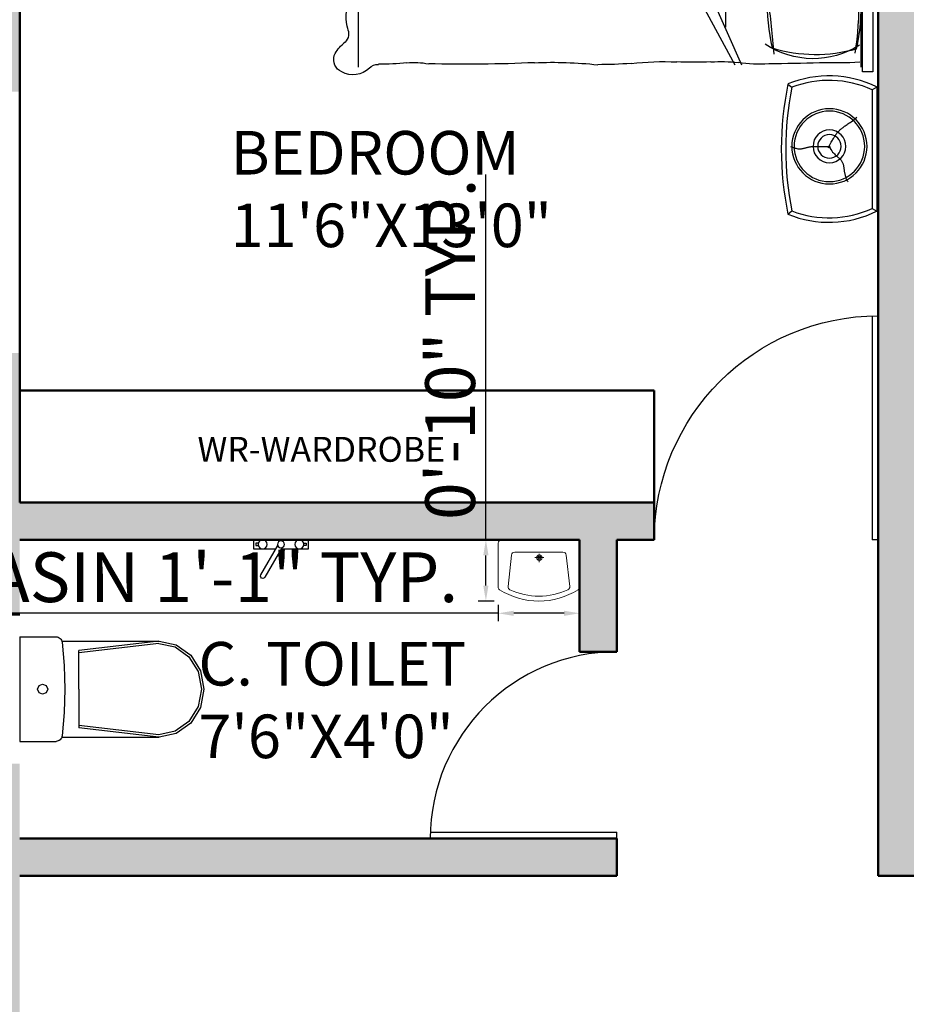
# Model space of a CAD drawing. Units: inches. Extents: x 1986 to 21484, y -1816 to 2016.
# Tile 7 of 85: x 2087 to 2230, y 1607 to 1765. Entities that reach past the tile are written whole.
import ezdxf

# ---------------------------------------------------------------- set-up
doc = ezdxf.new("R2010")
doc.units = ezdxf.units.IN
for name, color, linetype, lineweight in [('A-ANNO-DIMS', 2, 'Continuous', 18), ('A-ANNO-TEXT', 7, 'Continuous', 18), ('A-AREA-IDEN', 3, 'Continuous', 18), ('A-DOOR', 3, 'Continuous', 25), ('A-FLOR-FIXT', 8, 'Continuous', 18), ('A-FURN', 8, 'Continuous', 18), ('A-WALL', 7, 'Continuous', 50), ('A-WALL-PATT', 8, 'Continuous', 13)]:
    doc.layers.add(name, color=color, linetype=linetype, lineweight=lineweight)
doc.layers.add('SANTEH', color=7, linetype='Continuous')
doc.layers.add('TEFRİŞ', color=11, linetype='Continuous')
doc.styles.get("Standard").update_dxf_attribs({"font": 'arial.ttf'})
doc.dimstyles.new('ISO-25', dxfattribs={"dimtxt": 8, "dimasz": 2.5, "dimexe": 1.25, "dimexo": 0.625, "dimtad": 1, "dimdec": 1, "dimlunit": 3, "dimtxsty": 'Standard', "dimcen": 2.5, "dimadec": 0, "dimazin": 0, "dimtfac": 1, "dimtdec": 1, "dimtmove": 0, "dimatfit": 3, "dimfxl": 1, "dimarcsym": 0})

# ---------------------------------------------------------------- blocks, each defined once
blk = doc.blocks.new('D2')
for p, q in [((1722.5, 1505.46), (1722.5, 1475.46)), ((1723.5, 1505.46), (1723.5, 1475.46)), ((1722.5, 1475.46), (1723.5, 1475.46))]:
    blk.add_line(p, q)
blk.add_arc((1722.5, 1475.46), 30, 0, 90)
blk = doc.blocks.new('D1')
for p, q in [((1805.96, 1500.36), (1805.96, 1464.36)), ((1806.96, 1500.36), (1806.96, 1464.36)), ((1805.96, 1464.36), (1806.96, 1464.36))]:
    blk.add_line(p, q)
blk.add_arc((1805.96, 1464.36), 36, 0, 90)
blk = doc.blocks.new('WC 2 Symb_109')
at = {"layer": 'SANTEH'}
for p, q in [((0, 0), (0, 380)), ((0, 380), (132.4, 380)), ((153.6, 364.9), (506.8, 364.9)), ((506.3, 364.9), (215.7, 330.9)), ((506.3, 356), (215.7, 322)), ((215.7, 190), (215.7, 330.9)), ((215.7, 190), (215.7, 49.1)), ((506.3, 24), (215.7, 58)), ((506.3, 15.1), (215.7, 49.1)), ((153.8, 15.1), (506.8, 15.1)), ((0, 0), (132.4, 0))]:
    blk.add_line(p, q, dxfattribs=at)
for points in [[(154.6, 360.1), (153.9, 364.1), (152.3, 367.9), (150.2, 371.3), (147.4, 374.3), (144.1, 376.7), (140.5, 378.5), (136.5, 379.6), (132.4, 380)], [(154.6, 19.7), (158.6, 62.1), (161.4, 104.7), (163.1, 147.3), (163.7, 189.9), (163.1, 232.5), (161.4, 275.1), (158.6, 317.7), (154.6, 360.1)], [(506.8, 15.1), (569.2, 28.4), (622.2, 66.3), (657.6, 123.1), (670, 190), (657.6, 256.9), (622.2, 313.7), (569.2, 351.6), (506.8, 364.9)], [(506.3, 24), (565.5, 36.6), (615.7, 72.6), (649.2, 126.5), (661, 190), (649.2, 253.5), (615.7, 307.4), (565.5, 343.4), (506.3, 356)], [(132.4, 0), (136.5, 0.4), (140.4, 1.5), (144.1, 3.2), (147.3, 5.6), (150.1, 8.6), (152.3, 12), (153.8, 15.7), (154.6, 19.7)]]:
    blk.add_lwpolyline(points, dxfattribs=at)
blk.add_lwpolyline([(83.6, 208.5), (70.4, 203.1), (64.9, 190), (70.4, 176.9), (83.6, 171.5), (96.8, 176.9), (102.2, 190), (96.8, 203.1)], close=True, dxfattribs=at)
blk = doc.blocks.new('A$C2EBB240D')
for p, q in [((480, 375.8), (20, 375.8)), ((0, 355.8), (0, 86.6)), ((500, 355.8), (500, 86.6)), ((60.8, 89.8), (82.3, 282.2)), ((250, 300), (102.1, 300)), ((250, 300), (397.9, 300)), ((439.2, 89.8), (417.7, 282.2))]:
    blk.add_line(p, q)
for points in [[(275.2, 266.4), (219.4, 266.4)], [(247.3, 238.5), (247.3, 288.9)]]:
    blk.add_lwpolyline(points)
for centre, radius, start, end in [((20, 355.8), 20, 90, 180), ((480, 355.8), 20, 0, 90), ((102.1, 280), 20, 90, 173.64284), ((247.3, 266.4), 16.7, 90, 270), ((247.3, 266.4), 10, 90, 270), ((247.3, 266.4), 16.7, 270, 90), ((247.3, 266.4), 10, 270, 90), ((397.9, 280), 20, 6.35716, 90), ((20, 86.6), 20, 180, 237.68921), ((250, 450.3), 450.3, 237.68921, 270), ((80.7, 87.6), 20, 173.64284, 244.97956), ((250, 450.3), 420.3, 244.97956, 270), ((250, 450.3), 450.3, 270, 302.31079), ((250, 450.3), 420.3, 270, 295.02044), ((419.3, 87.6), 20, 295.02044, 6.35716), ((480, 86.6), 20, 302.31079, 0)]:
    blk.add_arc(centre, radius, start, end)
blk = doc.blocks.new('Faucet - kit sink top')
at = {"layer": 'SANTEH'}
for p, q in [((-5.5, -0.75), (-5.5, -1.25)), ((-4.94278, -0.75), (-5.5, -0.75)), ((-5.5, -1.25), (-4.94278, -1.25)), ((-0.14775, -1.7441), (3.56698, -8.1782)), ((4.43301, -7.6782), (0.71828, -1.2441)), ((4.94278, -0.75), (5.5, -0.75)), ((5.5, -1.25), (4.94278, -1.25)), ((5.5, -0.75), (5.5, -1.25))]:
    blk.add_line(p, q, dxfattribs=at)
blk.add_lwpolyline([(-0.00587, -2), (-6, -2), (-6, 0), (6, 0), (6, -2), (1.15195, -2)], dxfattribs=at)
for centre, radius in [((-4, -1), 1), ((4, -1), 1), ((0, -1), 0.75)]:
    blk.add_circle(centre, radius, dxfattribs=at)
blk.add_arc((4, -7.9282), 0.5, 210, 30, dxfattribs=at)
blk = doc.blocks.new('BED')
at = {"layer": 'TEFRİŞ'}
for p, q in [((2177.29, 1835.98), (2177.61, 1835.47)), ((2177.29, 1835.98), (2191.52, 1835.98)), ((2191.2, 1835.47), (2191.52, 1835.98)), ((2114.88, 1835.66), (2129.12, 1835.66)), ((2115.2, 1835.15), (2128.8, 1835.15)), ((2130.81, 1834.34), (2130.81, 1835.55)), ((2130.91, 1835.55), (2175.56, 1835.55)), ((2175.56, 1835.55), (2175.56, 1834.34)), ((2177.61, 1835.47), (2191.2, 1835.47)), ((2175.56, 1834.34), (2130.81, 1834.34)), ((2175, 1834.19), (2130.91, 1834.19)), ((2118.49, 1833.2), (2118.34, 1833.38)), ((2118.49, 1833.2), (2118.34, 1833.38)), ((2118.63, 1833.03), (2118.49, 1833.2)), ((2118.63, 1833.03), (2118.49, 1833.2)), ((2118.75, 1832.88), (2118.63, 1833.03)), ((2118.75, 1832.88), (2118.63, 1833.03)), ((2118.86, 1832.74), (2118.75, 1832.88)), ((2118.86, 1832.74), (2118.75, 1832.88)), ((2118.95, 1832.61), (2118.86, 1832.74)), ((2118.95, 1832.61), (2118.86, 1832.74)), ((2119.04, 1832.48), (2118.95, 1832.61)), ((2119.04, 1832.48), (2118.95, 1832.61)), ((2180.9, 1833.52), (2180.75, 1833.7)), ((2180.9, 1833.52), (2180.75, 1833.7)), ((2181.04, 1833.35), (2180.9, 1833.52)), ((2181.04, 1833.35), (2180.9, 1833.52)), ((2181.16, 1833.2), (2181.04, 1833.35)), ((2181.16, 1833.2), (2181.04, 1833.35)), ((2181.26, 1833.06), (2181.16, 1833.2)), ((2181.26, 1833.06), (2181.16, 1833.2)), ((2181.36, 1832.93), (2181.26, 1833.06)), ((2181.36, 1832.93), (2181.26, 1833.06)), ((2181.44, 1832.8), (2181.36, 1832.93)), ((2181.44, 1832.8), (2181.36, 1832.93)), ((2181.52, 1832.69), (2181.44, 1832.8)), ((2181.52, 1832.69), (2181.44, 1832.8)), ((2181.59, 1832.58), (2181.52, 1832.69)), ((2181.59, 1832.58), (2181.52, 1832.69)), ((2181.66, 1832.48), (2181.59, 1832.58)), ((2181.66, 1832.48), (2181.59, 1832.58)), ((2188.01, 1832.57), (2188.09, 1832.62)), ((2188.01, 1832.57), (2188.09, 1832.62)), ((2188.09, 1832.62), (2188.15, 1832.67)), ((2188.09, 1832.62), (2188.15, 1832.67)), ((2119.12, 1832.37), (2119.04, 1832.48)), ((2119.12, 1832.37), (2119.04, 1832.48)), ((2119.19, 1832.26), (2119.12, 1832.37)), ((2119.19, 1832.26), (2119.12, 1832.37)), ((2119.26, 1832.16), (2119.19, 1832.26)), ((2119.26, 1832.16), (2119.19, 1832.26)), ((2119.32, 1832.06), (2119.26, 1832.16)), ((2119.32, 1832.06), (2119.26, 1832.16)), ((2119.39, 1831.97), (2119.32, 1832.06)), ((2119.39, 1831.97), (2119.32, 1832.06)), ((2119.45, 1831.89), (2119.39, 1831.97)), ((2119.45, 1831.89), (2119.39, 1831.97)), ((2119.51, 1831.81), (2119.45, 1831.89)), ((2119.51, 1831.81), (2119.45, 1831.89)), ((2119.57, 1831.73), (2119.51, 1831.81)), ((2119.57, 1831.73), (2119.51, 1831.81)), ((2119.63, 1831.65), (2119.57, 1831.73)), ((2119.63, 1831.65), (2119.57, 1831.73)), ((2119.69, 1831.58), (2119.63, 1831.65)), ((2119.69, 1831.58), (2119.63, 1831.65)), ((2119.75, 1831.51), (2119.69, 1831.58)), ((2119.75, 1831.51), (2119.69, 1831.58)), ((2119.81, 1831.44), (2119.75, 1831.51)), ((2119.81, 1831.44), (2119.75, 1831.51)), ((2123.08, 1831.4), (2123.14, 1831.46)), ((2123.08, 1831.4), (2123.14, 1831.46)), ((2123.14, 1831.46), (2123.21, 1831.52)), ((2123.14, 1831.46), (2123.21, 1831.52)), ((2123.21, 1831.52), (2123.27, 1831.58)), ((2123.21, 1831.52), (2123.27, 1831.58)), ((2123.27, 1831.58), (2123.34, 1831.63)), ((2123.27, 1831.58), (2123.34, 1831.63)), ((2123.34, 1831.63), (2123.41, 1831.67)), ((2123.34, 1831.63), (2123.41, 1831.67)), ((2123.41, 1831.67), (2123.48, 1831.71)), ((2123.41, 1831.67), (2123.48, 1831.71)), ((2123.48, 1831.71), (2123.55, 1831.74)), ((2123.48, 1831.71), (2123.55, 1831.74)), ((2123.55, 1831.74), (2123.62, 1831.77)), ((2123.55, 1831.74), (2123.62, 1831.77)), ((2123.62, 1831.77), (2123.69, 1831.8)), ((2123.62, 1831.77), (2123.69, 1831.8)), ((2123.69, 1831.8), (2123.77, 1831.82)), ((2123.69, 1831.8), (2123.77, 1831.82)), ((2123.77, 1831.82), (2123.84, 1831.84)), ((2123.77, 1831.82), (2123.84, 1831.84)), ((2123.84, 1831.84), (2123.91, 1831.86)), ((2123.84, 1831.84), (2123.91, 1831.86)), ((2123.91, 1831.86), (2123.98, 1831.87)), ((2123.91, 1831.86), (2123.98, 1831.87)), ((2123.98, 1831.87), (2124.06, 1831.89)), ((2123.98, 1831.87), (2124.06, 1831.89)), ((2124.06, 1831.89), (2124.13, 1831.9)), ((2124.06, 1831.89), (2124.13, 1831.9)), ((2124.13, 1831.9), (2124.2, 1831.91)), ((2124.13, 1831.9), (2124.2, 1831.91)), ((2124.2, 1831.91), (2124.27, 1831.91)), ((2124.2, 1831.91), (2124.27, 1831.91)), ((2124.27, 1831.91), (2124.35, 1831.92)), ((2124.27, 1831.91), (2124.35, 1831.92)), ((2124.35, 1831.92), (2124.42, 1831.93)), ((2124.35, 1831.92), (2124.42, 1831.93)), ((2124.42, 1831.93), (2124.49, 1831.94)), ((2124.42, 1831.93), (2124.49, 1831.94)), ((2124.49, 1831.94), (2124.56, 1831.95)), ((2124.49, 1831.94), (2124.56, 1831.95)), ((2124.56, 1831.95), (2124.64, 1831.96)), ((2124.56, 1831.95), (2124.64, 1831.96)), ((2124.64, 1831.96), (2124.71, 1831.98)), ((2124.64, 1831.96), (2124.71, 1831.98)), ((2124.71, 1831.98), (2124.79, 1831.99)), ((2124.71, 1831.98), (2124.79, 1831.99)), ((2124.79, 1831.99), (2124.87, 1832.01)), ((2124.79, 1831.99), (2124.87, 1832.01)), ((2124.87, 1832.01), (2124.96, 1832.03)), ((2124.87, 1832.01), (2124.96, 1832.03)), ((2124.96, 1832.03), (2125.05, 1832.05)), ((2124.96, 1832.03), (2125.05, 1832.05)), ((2125.05, 1832.05), (2125.14, 1832.08)), ((2125.05, 1832.05), (2125.14, 1832.08)), ((2125.14, 1832.08), (2125.23, 1832.11)), ((2125.14, 1832.08), (2125.23, 1832.11)), ((2125.23, 1832.11), (2125.33, 1832.14)), ((2125.23, 1832.11), (2125.33, 1832.14)), ((2125.33, 1832.14), (2125.42, 1832.17)), ((2125.33, 1832.14), (2125.42, 1832.17)), ((2125.42, 1832.17), (2125.52, 1832.21)), ((2125.42, 1832.17), (2125.52, 1832.21)), ((2125.52, 1832.21), (2125.6, 1832.25)), ((2125.52, 1832.21), (2125.6, 1832.25)), ((2125.6, 1832.25), (2125.68, 1832.3)), ((2125.6, 1832.25), (2125.68, 1832.3)), ((2125.68, 1832.3), (2125.75, 1832.35)), ((2125.68, 1832.3), (2125.75, 1832.35)), ((2181.73, 1832.38), (2181.66, 1832.48)), ((2181.73, 1832.38), (2181.66, 1832.48)), ((2181.79, 1832.29), (2181.73, 1832.38)), ((2181.79, 1832.29), (2181.73, 1832.38)), ((2181.85, 1832.21), (2181.79, 1832.29)), ((2181.85, 1832.21), (2181.79, 1832.29)), ((2181.92, 1832.13), (2181.85, 1832.21)), ((2181.92, 1832.13), (2181.85, 1832.21)), ((2181.97, 1832.05), (2181.92, 1832.13)), ((2181.97, 1832.05), (2181.92, 1832.13)), ((2182.03, 1831.97), (2181.97, 1832.05)), ((2182.03, 1831.97), (2181.97, 1832.05)), ((2182.09, 1831.9), (2182.03, 1831.97)), ((2182.09, 1831.9), (2182.03, 1831.97)), ((2182.15, 1831.83), (2182.09, 1831.9)), ((2182.15, 1831.83), (2182.09, 1831.9)), ((2182.21, 1831.76), (2182.15, 1831.83)), ((2182.21, 1831.76), (2182.15, 1831.83)), ((2182.27, 1831.7), (2182.21, 1831.76)), ((2182.27, 1831.7), (2182.21, 1831.76)), ((2182.33, 1831.63), (2182.27, 1831.7)), ((2182.33, 1831.63), (2182.27, 1831.7)), ((2182.4, 1831.57), (2182.33, 1831.63)), ((2182.4, 1831.57), (2182.33, 1831.63)), ((2182.46, 1831.52), (2182.4, 1831.57)), ((2182.46, 1831.52), (2182.4, 1831.57)), ((2182.52, 1831.46), (2182.46, 1831.52)), ((2182.52, 1831.46), (2182.46, 1831.52)), ((2182.59, 1831.41), (2182.52, 1831.46)), ((2182.59, 1831.41), (2182.52, 1831.46)), ((2185.21, 1831.41), (2185.28, 1831.5)), ((2185.21, 1831.41), (2185.28, 1831.5)), ((2185.28, 1831.5), (2185.35, 1831.58)), ((2185.28, 1831.5), (2185.35, 1831.58)), ((2185.35, 1831.58), (2185.42, 1831.65)), ((2185.35, 1831.58), (2185.42, 1831.65)), ((2185.42, 1831.65), (2185.48, 1831.72)), ((2185.42, 1831.65), (2185.48, 1831.72)), ((2185.48, 1831.72), (2185.55, 1831.78)), ((2185.48, 1831.72), (2185.55, 1831.78)), ((2185.55, 1831.78), (2185.61, 1831.84)), ((2185.55, 1831.78), (2185.61, 1831.84)), ((2185.61, 1831.84), (2185.68, 1831.9)), ((2185.61, 1831.84), (2185.68, 1831.9)), ((2185.68, 1831.9), (2185.75, 1831.95)), ((2185.68, 1831.9), (2185.75, 1831.95)), ((2185.75, 1831.95), (2185.82, 1831.99)), ((2185.75, 1831.95), (2185.82, 1831.99)), ((2185.82, 1831.99), (2185.89, 1832.03)), ((2185.82, 1831.99), (2185.89, 1832.03)), ((2185.89, 1832.03), (2185.96, 1832.06)), ((2185.89, 1832.03), (2185.96, 1832.06)), ((2185.96, 1832.06), (2186.03, 1832.09)), ((2185.96, 1832.06), (2186.03, 1832.09)), ((2186.03, 1832.09), (2186.1, 1832.12)), ((2186.03, 1832.09), (2186.1, 1832.12)), ((2186.1, 1832.12), (2186.17, 1832.14)), ((2186.1, 1832.12), (2186.17, 1832.14)), ((2186.17, 1832.14), (2186.24, 1832.16)), ((2186.17, 1832.14), (2186.24, 1832.16)), ((2186.24, 1832.16), (2186.32, 1832.18)), ((2186.24, 1832.16), (2186.32, 1832.18)), ((2186.32, 1832.18), (2186.39, 1832.19)), ((2186.32, 1832.18), (2186.39, 1832.19)), ((2186.39, 1832.19), (2186.46, 1832.21)), ((2186.39, 1832.19), (2186.46, 1832.21)), ((2186.46, 1832.21), (2186.53, 1832.22)), ((2186.46, 1832.21), (2186.53, 1832.22)), ((2186.53, 1832.22), (2186.61, 1832.23)), ((2186.53, 1832.22), (2186.61, 1832.23)), ((2186.61, 1832.23), (2186.68, 1832.23)), ((2186.61, 1832.23), (2186.68, 1832.23)), ((2186.68, 1832.23), (2186.75, 1832.24)), ((2186.68, 1832.23), (2186.75, 1832.24)), ((2186.75, 1832.24), (2186.82, 1832.25)), ((2186.75, 1832.24), (2186.82, 1832.25)), ((2186.82, 1832.25), (2186.9, 1832.26)), ((2186.82, 1832.25), (2186.9, 1832.26)), ((2186.9, 1832.26), (2186.97, 1832.27)), ((2186.9, 1832.26), (2186.97, 1832.27)), ((2186.97, 1832.27), (2187.04, 1832.28)), ((2186.97, 1832.27), (2187.04, 1832.28)), ((2187.04, 1832.28), (2187.12, 1832.3)), ((2187.04, 1832.28), (2187.12, 1832.3)), ((2187.12, 1832.3), (2187.2, 1832.31)), ((2187.12, 1832.3), (2187.2, 1832.31)), ((2187.2, 1832.31), (2187.28, 1832.33)), ((2187.2, 1832.31), (2187.28, 1832.33)), ((2187.28, 1832.33), (2187.36, 1832.35)), ((2187.28, 1832.33), (2187.36, 1832.35)), ((2187.36, 1832.35), (2187.45, 1832.37)), ((2187.36, 1832.35), (2187.45, 1832.37)), ((2187.45, 1832.37), (2187.54, 1832.4)), ((2187.45, 1832.37), (2187.54, 1832.4)), ((2187.54, 1832.4), (2187.64, 1832.43)), ((2187.54, 1832.4), (2187.64, 1832.43)), ((2187.64, 1832.43), (2187.74, 1832.46)), ((2187.64, 1832.43), (2187.74, 1832.46)), ((2187.74, 1832.46), (2187.83, 1832.49)), ((2187.74, 1832.46), (2187.83, 1832.49)), ((2187.83, 1832.49), (2187.92, 1832.53)), ((2187.83, 1832.49), (2187.92, 1832.53)), ((2187.92, 1832.53), (2188.01, 1832.57)), ((2187.92, 1832.53), (2188.01, 1832.57)), ((2119.87, 1831.38), (2119.81, 1831.44)), ((2119.87, 1831.38), (2119.81, 1831.44)), ((2119.93, 1831.31), (2119.87, 1831.38)), ((2119.93, 1831.31), (2119.87, 1831.38)), ((2119.99, 1831.25), (2119.93, 1831.31)), ((2119.99, 1831.25), (2119.93, 1831.31)), ((2120.05, 1831.2), (2119.99, 1831.25)), ((2120.05, 1831.2), (2119.99, 1831.25)), ((2120.12, 1831.14), (2120.05, 1831.2)), ((2120.12, 1831.14), (2120.05, 1831.2)), ((2120.18, 1831.09), (2120.12, 1831.14)), ((2120.18, 1831.09), (2120.12, 1831.14)), ((2120.25, 1831.04), (2120.18, 1831.09)), ((2120.25, 1831.04), (2120.18, 1831.09)), ((2120.32, 1830.99), (2120.25, 1831.04)), ((2120.32, 1830.99), (2120.25, 1831.04)), ((2120.39, 1830.94), (2120.32, 1830.99)), ((2120.39, 1830.94), (2120.32, 1830.99)), ((2120.47, 1830.9), (2120.39, 1830.94)), ((2120.47, 1830.9), (2120.39, 1830.94)), ((2120.54, 1830.85), (2120.47, 1830.9)), ((2120.54, 1830.85), (2120.47, 1830.9)), ((2120.62, 1830.8), (2120.54, 1830.85)), ((2120.62, 1830.8), (2120.54, 1830.85)), ((2120.7, 1830.75), (2120.62, 1830.8)), ((2120.7, 1830.75), (2120.62, 1830.8)), ((2120.79, 1830.7), (2120.7, 1830.75)), ((2120.79, 1830.7), (2120.7, 1830.75)), ((2120.88, 1830.65), (2120.79, 1830.7)), ((2120.88, 1830.65), (2120.79, 1830.7)), ((2120.98, 1830.59), (2120.88, 1830.65)), ((2120.98, 1830.59), (2120.88, 1830.65)), ((2121.09, 1830.52), (2120.98, 1830.59)), ((2121.09, 1830.52), (2120.98, 1830.59)), ((2121.21, 1830.45), (2121.09, 1830.52)), ((2121.21, 1830.45), (2121.09, 1830.52)), ((2121.34, 1830.38), (2121.21, 1830.45)), ((2121.34, 1830.38), (2121.21, 1830.45)), ((2121.49, 1830.29), (2121.34, 1830.38)), ((2121.49, 1830.29), (2121.34, 1830.38)), ((2121.76, 1830.38), (2121.74, 1830.17)), ((2121.76, 1830.38), (2121.74, 1830.17)), ((2121.87, 1830.29), (2122.04, 1830.4)), ((2121.87, 1830.29), (2122.04, 1830.4)), ((2122.04, 1830.4), (2122.2, 1830.51)), ((2122.04, 1830.4), (2122.2, 1830.51)), ((2122.2, 1830.51), (2122.33, 1830.61)), ((2122.2, 1830.51), (2122.33, 1830.61)), ((2122.33, 1830.61), (2122.45, 1830.72)), ((2122.33, 1830.61), (2122.45, 1830.72)), ((2122.45, 1830.72), (2122.55, 1830.82)), ((2122.45, 1830.72), (2122.55, 1830.82)), ((2122.55, 1830.82), (2122.64, 1830.91)), ((2122.55, 1830.82), (2122.64, 1830.91)), ((2122.64, 1830.91), (2122.72, 1831.01)), ((2122.64, 1830.91), (2122.72, 1831.01)), ((2122.72, 1831.01), (2122.8, 1831.09)), ((2122.72, 1831.01), (2122.8, 1831.09)), ((2122.8, 1831.09), (2122.87, 1831.18)), ((2122.8, 1831.09), (2122.87, 1831.18)), ((2122.87, 1831.18), (2122.94, 1831.26)), ((2122.87, 1831.18), (2122.94, 1831.26)), ((2122.94, 1831.26), (2123.01, 1831.33)), ((2122.94, 1831.26), (2123.01, 1831.33)), ((2123.01, 1831.33), (2123.08, 1831.4)), ((2123.01, 1831.33), (2123.08, 1831.4)), ((2182.66, 1831.36), (2182.59, 1831.41)), ((2182.66, 1831.36), (2182.59, 1831.41)), ((2182.73, 1831.31), (2182.66, 1831.36)), ((2182.73, 1831.31), (2182.66, 1831.36)), ((2182.8, 1831.26), (2182.73, 1831.31)), ((2182.8, 1831.26), (2182.73, 1831.31)), ((2182.87, 1831.22), (2182.8, 1831.26)), ((2182.87, 1831.22), (2182.8, 1831.26)), ((2182.95, 1831.17), (2182.87, 1831.22)), ((2182.95, 1831.17), (2182.87, 1831.22)), ((2183.03, 1831.12), (2182.95, 1831.17)), ((2183.03, 1831.12), (2182.95, 1831.17)), ((2183.11, 1831.07), (2183.03, 1831.12)), ((2183.11, 1831.07), (2183.03, 1831.12)), ((2183.2, 1831.02), (2183.11, 1831.07)), ((2183.2, 1831.02), (2183.11, 1831.07)), ((2183.29, 1830.97), (2183.2, 1831.02)), ((2183.29, 1830.97), (2183.2, 1831.02)), ((2183.39, 1830.91), (2183.29, 1830.97)), ((2183.39, 1830.91), (2183.29, 1830.97)), ((2183.49, 1830.84), (2183.39, 1830.91)), ((2183.49, 1830.84), (2183.39, 1830.91)), ((2183.61, 1830.77), (2183.49, 1830.84)), ((2183.61, 1830.77), (2183.49, 1830.84)), ((2183.75, 1830.7), (2183.61, 1830.77)), ((2183.75, 1830.7), (2183.61, 1830.77)), ((2183.9, 1830.61), (2183.75, 1830.7)), ((2183.9, 1830.61), (2183.75, 1830.7)), ((2184.06, 1830.53), (2183.9, 1830.61)), ((2184.06, 1830.53), (2183.9, 1830.61)), ((2184.25, 1830.43), (2184.06, 1830.53)), ((2184.25, 1830.43), (2184.06, 1830.53)), ((2184.07, 1830.5), (2184.27, 1830.61)), ((2184.07, 1830.5), (2184.27, 1830.61)), ((2184.15, 1830.49), (2184.14, 1830.31)), ((2184.15, 1830.49), (2184.14, 1830.31)), ((2184.17, 1830.7), (2184.15, 1830.49)), ((2184.17, 1830.7), (2184.15, 1830.49)), ((2184.27, 1830.61), (2184.45, 1830.72)), ((2184.27, 1830.61), (2184.45, 1830.72)), ((2184.45, 1830.72), (2184.6, 1830.83)), ((2184.45, 1830.72), (2184.6, 1830.83)), ((2184.6, 1830.83), (2184.74, 1830.93)), ((2184.6, 1830.83), (2184.74, 1830.93)), ((2184.74, 1830.93), (2184.85, 1831.04)), ((2184.74, 1830.93), (2184.85, 1831.04)), ((2184.85, 1831.04), (2184.95, 1831.14)), ((2184.85, 1831.04), (2184.95, 1831.14)), ((2184.95, 1831.14), (2185.05, 1831.23)), ((2184.95, 1831.14), (2185.05, 1831.23)), ((2185.05, 1831.23), (2185.13, 1831.33)), ((2185.05, 1831.23), (2185.13, 1831.33)), ((2185.13, 1831.33), (2185.21, 1831.41)), ((2185.13, 1831.33), (2185.21, 1831.41)), ((2121.66, 1830.21), (2121.49, 1830.29)), ((2121.66, 1830.21), (2121.49, 1830.29)), ((2121.66, 1830.18), (2121.87, 1830.29)), ((2121.66, 1830.18), (2121.87, 1830.29)), ((2121.85, 1830.11), (2121.66, 1830.21)), ((2121.85, 1830.11), (2121.66, 1830.21)), ((2121.74, 1829.99), (2121.73, 1829.83)), ((2121.74, 1829.99), (2121.73, 1829.83)), ((2121.73, 1829.83), (2121.73, 1829.69)), ((2121.73, 1829.83), (2121.73, 1829.69)), ((2121.73, 1829.69), (2121.73, 1829.57)), ((2121.73, 1829.69), (2121.73, 1829.57)), ((2121.73, 1829.57), (2121.73, 1829.45)), ((2121.73, 1829.57), (2121.73, 1829.45)), ((2121.73, 1829.45), (2121.74, 1829.35)), ((2121.73, 1829.45), (2121.74, 1829.35)), ((2121.74, 1830.17), (2121.74, 1829.99)), ((2121.74, 1830.17), (2121.74, 1829.99)), ((2121.74, 1829.35), (2121.74, 1829.25)), ((2121.74, 1829.35), (2121.74, 1829.25)), ((2121.74, 1829.25), (2121.74, 1829.16)), ((2121.74, 1829.25), (2121.74, 1829.16)), ((2184.14, 1830.31), (2184.14, 1830.15)), ((2184.14, 1830.31), (2184.14, 1830.15)), ((2184.14, 1830.15), (2184.14, 1830.01)), ((2184.14, 1830.15), (2184.14, 1830.01)), ((2184.14, 1830.01), (2184.14, 1829.89)), ((2184.14, 1830.01), (2184.14, 1829.89)), ((2184.14, 1829.89), (2184.14, 1829.77)), ((2184.14, 1829.89), (2184.14, 1829.77)), ((2184.14, 1829.77), (2184.14, 1829.67)), ((2184.14, 1829.77), (2184.14, 1829.67)), ((2184.14, 1829.67), (2184.15, 1829.57)), ((2184.14, 1829.67), (2184.15, 1829.57)), ((2184.15, 1829.38), (2184.14, 1829.29)), ((2184.15, 1829.38), (2184.14, 1829.29)), ((2184.14, 1829.29), (2184.14, 1829.21)), ((2184.14, 1829.29), (2184.14, 1829.21)), ((2184.14, 1829.21), (2184.14, 1829.12)), ((2184.14, 1829.21), (2184.14, 1829.12)), ((2184.15, 1829.57), (2184.15, 1829.48)), ((2184.15, 1829.57), (2184.15, 1829.48)), ((2184.15, 1829.48), (2184.15, 1829.38)), ((2184.15, 1829.48), (2184.15, 1829.38)), ((2121.74, 1828.89), (2121.73, 1828.8)), ((2121.74, 1828.89), (2121.73, 1828.8)), ((2121.73, 1828.8), (2121.73, 1828.72)), ((2121.73, 1828.8), (2121.73, 1828.72)), ((2121.73, 1828.72), (2121.73, 1828.64)), ((2121.73, 1828.72), (2121.73, 1828.64)), ((2121.73, 1828.64), (2121.73, 1828.56)), ((2121.73, 1828.64), (2121.73, 1828.56)), ((2121.73, 1828.56), (2121.73, 1828.48)), ((2121.73, 1828.56), (2121.73, 1828.48)), ((2121.73, 1828.48), (2121.73, 1828.4)), ((2121.73, 1828.48), (2121.73, 1828.4)), ((2121.73, 1828.4), (2121.73, 1828.33)), ((2121.73, 1828.4), (2121.73, 1828.33)), ((2121.73, 1828.33), (2121.74, 1828.25)), ((2121.73, 1828.33), (2121.74, 1828.25)), ((2121.74, 1829.16), (2121.74, 1829.06)), ((2121.74, 1829.16), (2121.74, 1829.06)), ((2121.74, 1829.06), (2121.74, 1828.97)), ((2121.74, 1829.06), (2121.74, 1828.97)), ((2121.74, 1828.97), (2121.74, 1828.89)), ((2121.74, 1828.97), (2121.74, 1828.89)), ((2121.74, 1828.25), (2121.75, 1828.18)), ((2121.74, 1828.25), (2121.75, 1828.18)), ((2121.75, 1828.18), (2121.75, 1828.1)), ((2121.75, 1828.18), (2121.75, 1828.1)), ((2121.75, 1828.1), (2121.76, 1828.03)), ((2121.75, 1828.1), (2121.76, 1828.03)), ((2184.14, 1829.04), (2184.13, 1828.96)), ((2184.14, 1829.04), (2184.13, 1828.96)), ((2184.13, 1828.96), (2184.13, 1828.88)), ((2184.13, 1828.96), (2184.13, 1828.88)), ((2184.13, 1828.88), (2184.13, 1828.8)), ((2184.13, 1828.88), (2184.13, 1828.8)), ((2184.13, 1828.8), (2184.14, 1828.72)), ((2184.13, 1828.8), (2184.14, 1828.72)), ((2184.14, 1829.12), (2184.14, 1829.04)), ((2184.14, 1829.12), (2184.14, 1829.04)), ((2184.14, 1828.72), (2184.14, 1828.65)), ((2184.14, 1828.72), (2184.14, 1828.65)), ((2184.14, 1828.65), (2184.15, 1828.57)), ((2184.14, 1828.65), (2184.15, 1828.57)), ((2184.15, 1828.57), (2184.15, 1828.5)), ((2184.15, 1828.57), (2184.15, 1828.5)), ((2184.15, 1828.5), (2184.16, 1828.42)), ((2184.15, 1828.5), (2184.16, 1828.42)), ((2184.16, 1828.42), (2184.17, 1828.35)), ((2184.16, 1828.42), (2184.17, 1828.35)), ((2184.17, 1828.35), (2184.18, 1828.27)), ((2184.17, 1828.35), (2184.18, 1828.27)), ((2184.18, 1828.27), (2184.19, 1828.2)), ((2184.18, 1828.27), (2184.19, 1828.2)), ((2184.19, 1828.2), (2184.21, 1828.12)), ((2184.19, 1828.2), (2184.21, 1828.12)), ((2184.21, 1828.12), (2184.22, 1828.04)), ((2184.21, 1828.12), (2184.22, 1828.04)), ((2121.76, 1828.03), (2121.78, 1827.95)), ((2121.76, 1828.03), (2121.78, 1827.95)), ((2121.78, 1827.95), (2121.79, 1827.88)), ((2121.78, 1827.95), (2121.79, 1827.88)), ((2121.79, 1827.88), (2121.8, 1827.8)), ((2121.79, 1827.88), (2121.8, 1827.8)), ((2121.8, 1827.8), (2121.82, 1827.72)), ((2121.8, 1827.8), (2121.82, 1827.72)), ((2121.82, 1827.72), (2121.84, 1827.65)), ((2121.82, 1827.72), (2121.84, 1827.65)), ((2121.84, 1827.65), (2121.85, 1827.57)), ((2121.84, 1827.65), (2121.85, 1827.57)), ((2121.85, 1827.57), (2121.87, 1827.49)), ((2121.85, 1827.57), (2121.87, 1827.49)), ((2121.87, 1827.49), (2121.89, 1827.41)), ((2121.87, 1827.49), (2121.89, 1827.41)), ((2121.89, 1827.41), (2121.91, 1827.33)), ((2121.89, 1827.41), (2121.91, 1827.33)), ((2121.91, 1827.33), (2121.93, 1827.26)), ((2121.91, 1827.33), (2121.93, 1827.26)), ((2121.93, 1827.26), (2121.95, 1827.18)), ((2121.93, 1827.26), (2121.95, 1827.18)), ((2121.95, 1827.18), (2121.97, 1827.09)), ((2121.95, 1827.18), (2121.97, 1827.09)), ((2121.97, 1827.09), (2121.99, 1827.01)), ((2121.97, 1827.09), (2121.99, 1827.01)), ((2121.99, 1827.01), (2122, 1826.93)), ((2121.99, 1827.01), (2122, 1826.93)), ((2184.22, 1828.04), (2184.24, 1827.97)), ((2184.22, 1828.04), (2184.24, 1827.97)), ((2184.24, 1827.97), (2184.26, 1827.89)), ((2184.24, 1827.97), (2184.26, 1827.89)), ((2184.26, 1827.89), (2184.28, 1827.81)), ((2184.26, 1827.89), (2184.28, 1827.81)), ((2184.28, 1827.81), (2184.3, 1827.73)), ((2184.28, 1827.81), (2184.3, 1827.73)), ((2184.3, 1827.73), (2184.32, 1827.65)), ((2184.3, 1827.73), (2184.32, 1827.65)), ((2184.32, 1827.65), (2184.34, 1827.58)), ((2184.32, 1827.65), (2184.34, 1827.58)), ((2184.34, 1827.58), (2184.36, 1827.5)), ((2184.34, 1827.58), (2184.36, 1827.5)), ((2184.36, 1827.5), (2184.38, 1827.41)), ((2184.36, 1827.5), (2184.38, 1827.41)), ((2184.38, 1827.41), (2184.4, 1827.33)), ((2184.38, 1827.41), (2184.4, 1827.33)), ((2184.4, 1826.96), (2184.38, 1826.86)), ((2184.4, 1826.96), (2184.38, 1826.86)), ((2184.4, 1827.33), (2184.41, 1827.25)), ((2184.4, 1827.33), (2184.41, 1827.25)), ((2184.41, 1827.06), (2184.4, 1826.96)), ((2184.41, 1827.06), (2184.4, 1826.96)), ((2184.41, 1827.25), (2184.41, 1827.16)), ((2184.41, 1827.25), (2184.41, 1827.16)), ((2184.41, 1827.16), (2184.41, 1827.06)), ((2184.41, 1827.16), (2184.41, 1827.06)), ((2121.78, 1825.93), (2121.74, 1825.8)), ((2121.78, 1825.93), (2121.74, 1825.8)), ((2121.83, 1826.06), (2121.78, 1825.93)), ((2121.83, 1826.06), (2121.78, 1825.93)), ((2121.87, 1826.19), (2121.83, 1826.06)), ((2121.87, 1826.19), (2121.83, 1826.06)), ((2121.91, 1826.31), (2121.87, 1826.19)), ((2121.91, 1826.31), (2121.87, 1826.19)), ((2121.95, 1826.42), (2121.91, 1826.31)), ((2121.95, 1826.42), (2121.91, 1826.31)), ((2121.97, 1826.54), (2121.95, 1826.42)), ((2121.97, 1826.54), (2121.95, 1826.42)), ((2121.99, 1826.64), (2121.97, 1826.54)), ((2121.99, 1826.64), (2121.97, 1826.54)), ((2122, 1826.74), (2121.99, 1826.64)), ((2122, 1826.74), (2121.99, 1826.64)), ((2122, 1826.93), (2122.01, 1826.84)), ((2122, 1826.93), (2122.01, 1826.84)), ((2122.01, 1826.84), (2122, 1826.74)), ((2122.01, 1826.84), (2122, 1826.74)), ((2129.46, 1825.49), (2129.09, 1825.93)), ((2176.94, 1825.81), (2177.31, 1826.25)), ((2184.19, 1826.25), (2184.14, 1826.12)), ((2184.19, 1826.25), (2184.14, 1826.12)), ((2184.23, 1826.38), (2184.19, 1826.25)), ((2184.23, 1826.38), (2184.19, 1826.25)), ((2184.28, 1826.51), (2184.23, 1826.38)), ((2184.28, 1826.51), (2184.23, 1826.38)), ((2184.32, 1826.63), (2184.28, 1826.51)), ((2184.32, 1826.63), (2184.28, 1826.51)), ((2184.35, 1826.74), (2184.32, 1826.63)), ((2184.35, 1826.74), (2184.32, 1826.63)), ((2184.38, 1826.86), (2184.35, 1826.74)), ((2184.38, 1826.86), (2184.35, 1826.74)), ((2191.87, 1825.81), (2191.5, 1826.25)), ((2174.77, 1820.53), (2130.76, 1800.91)), ((2174.77, 1819.77), (2130.6, 1795.83)), ((2140.43, 1818.69), (2131.53, 1818.69)), ((2157.71, 1818.69), (2156.77, 1818.69)), ((2170.41, 1818.69), (2164.92, 1818.69)), ((2141.43, 1817.4), (2131.53, 1817.4)), ((2149.62, 1817.4), (2145.88, 1817.4)), ((2167.36, 1817.4), (2154.77, 1817.4)), ((2175, 1776.57), (2130.11, 1776.57)), ((2138.52, 1775.41), (2167.39, 1775.41))]:
    blk.add_line(p, q, dxfattribs=at)
for centre, radius, start, end in [((2188.4, 1830.51), 12.39, 153.8162, 202.314), ((2180.41, 1830.51), 12.39, 337.686, 26.1838), ((2126, 1830.19), 12.39, 153.8162, 202.314), ((2126, 1830.19), 11.88, 155.3335, 201.0157), ((2118, 1830.19), 11.88, 338.9843, 24.6665), ((2118, 1830.19), 12.39, 337.686, 26.1838), ((2188.4, 1830.51), 11.88, 155.3335, 201.0157), ((2180.41, 1830.51), 11.88, 338.9843, 24.6665), ((2122, 1861.35), 36.12, 258.6773, 281.3227), ((2184.41, 1861.67), 36.63, 258.2443, 281.7557), ((2184.41, 1861.67), 36.12, 258.6773, 281.3227), ((2122, 1861.35), 36.63, 258.2443, 281.7557)]:
    blk.add_arc(centre, radius, start, end, dxfattribs=at)
at = {"layer": 'TEFRİŞ', "extrusion": (0, 0, -1)}
for centre, major_axis, ratio, start_param, end_param in [((2184.09, 1830.56), (-3.05, -3.05), 1, 3.926991, 10.210176), ((2184.09, 1830.56), (2.86, -2.86), 1, 5.497787, 11.780972), ((2184.09, 1830.56), (2.86, -2.86), 1, 5.497787, 11.780972), ((2121.68, 1830.24), (-3.05, -3.05), 1, 3.926991, 10.210176), ((2121.68, 1830.24), (2.86, -2.86), 1, 5.497787, 11.780972), ((2121.68, 1830.24), (2.86, -2.86), 1, 5.497787, 11.780972), ((2139.43, 1773.84), (-42.35, 42.35), 1, 0.646251, 0.896949), ((2206.14, 1830.73), (-52.86, -52.86), 1, 0.767743, 0.83177), ((2138.85, 1803.05), (-22.1, 22.1), 1, 0.544604, 1.006234), ((2181.61, 1828.44), (-34.39, 34.39), 1, -0.888486, -0.672463), ((2164.51, 1832.79), (-13.41, 13.41), 1, -0.974476, -0.730892), ((2154.12, 1796.61), (-26.46, 26.46), 1, 0.596409, 0.940188), ((2183.72, 1833.22), (-17, 17), 1, -0.967105, -0.749712), ((2168.35, 1789.27), (-1.33, 44.62), 0.875277, -0.163954, 0.163954), ((2087.32, 1833.96), (-52.37, 52.37), 1, 2.358049, 2.431787), ((2167.6, 1797.72), (-0.51, 36.47), 0.865194, -0.185965, 0.185965), ((2164.15, 1828.7), (-6.99, 6.99), 1, 1.789136, 2.946702), ((2099.77, 1830.73), (-52.86, 52.86), 1, 2.311571, 2.373849), ((2154.7, 1828.89), (-15.68, 15.68), 1, -1.00675, -0.580436), ((2127.6, 1828.81), (-13.23, 13.23), 1, 2.100388, 2.328052), ((2155, 1761.9), (-50.65, -50.65), 1, 2.239512, 2.426533), ((2172.01, 1828.66), (-17.93, 17.93), 1, -0.753394, -0.598744), ((2128.44, 1832.96), (-13.26, -13.26), 1, 3.889049, 4.127298), ((2134, 1828.8), (-18.62, 18.62), 1, 2.173461, 2.355043), ((2199.2, 1828.45), (-27.06, -27.06), 1, 0.770625, 0.917228), ((2156.76, 1828.98), (-11.9, -11.9), 1, 3.646453, 4.226155), ((2121.68, 1830.24), (1.33, -1.33), 1, 5.497787, 11.780972), ((2121.68, 1830.24), (1.33, -1.33), 1, 5.497787, 11.780972), ((2121.68, 1830.24), (0.952, -0.952), 1, 5.497787, 11.780972), ((2121.68, 1830.24), (0.952, -0.952), 1, 5.497787, 11.780972), ((2184.09, 1830.56), (1.33, -1.33), 1, 5.497787, 11.780972), ((2184.09, 1830.56), (1.33, -1.33), 1, 5.497787, 11.780972), ((2184.09, 1830.56), (0.952, -0.952), 1, 5.497787, 11.780972), ((2184.09, 1830.56), (0.952, -0.952), 1, 5.497787, 11.780972), ((2159.55, 1823.33), (-5.81, 5.81), 1, -0.516587, 0.256776), ((2154.84, 1827.75), (-1.93, 1.93), 1, 0.997904, 1.977819), ((2675.38, 1815.09), (-384.79, -384.79), 1, 0.80103, 0.811711), ((2166.67, 1824.96), (-2.93, 3.91), 0.760601, -0.723751, 0.723751), ((2153.88, 1825.05), (-9.22, 9.22), 1, 1.994956, 2.818753), ((1630.53, 1815.09), (-384.79, 384.79), 1, 2.329881, 2.340562), ((2147.44, 1824.41), (-3.36, -3.36), 1, 1.11934, 2.270556), ((2145.66, 1827.01), (-1.62, 1.62), 1, 1.310976, 2.284591), ((2172, 1826.44), (-11.23, 11.23), 1, -1.332486, -0.624868), ((2158.82, 1823.55), (-3.74, -3.74), 1, 1.730792, 3.47045), ((2157.83, 1821.53), (-4.47, 4.47), 1, 0.576679, 2.021689), ((2140.05, 1819.86), (-5.1, 5.1), 1, 0.238357, 1.390139), ((2139.42, 1820.79), (-4.21, -4.21), 1, 1.82161, 3.349145), ((2160.6, 1825.98), (-9.68, -9.68), 1, 0.009196, 0.886853), ((2148.35, 1820.65), (-4.63, -4.63), 1, 2.117602, 3.020837), ((2147.86, 1820.64), (-4.48, 4.48), 1, 0.665914, 1.867503), ((2141.71, 1819.83), (-11.86, 11.86), 1, 1.850844, 2.42862), ((2148.15, 1825.25), (-7.14, -7.14), 1, 6.061986, 7.190757), ((2154.93, 1828.48), (-11.96, 11.96), 1, -1.530302, -0.934407), ((2170.68, 1829.67), (-16.79, 16.79), 1, -1.354718, -0.902276), ((2127.37, 1815.76), (-10.68, 10.68), 1, 1.657204, 1.779381), ((2146.08, 1822.57), (-10.5, 10.5), 1, -0.951783, -0.716225), ((2132.43, 1774.09), (-35.41, -35.41), 1, 2.362911, 2.464592), ((2140.17, 1862.96), (-27.99, 27.99), 1, 3.983025, 4.107469), ((2165.73, 1860.69), (-26.41, -26.41), 1, 5.306413, 5.463767), ((2199.62, 1529.47), (-209.2, 209.2), 1, 0.675361, 0.697001), ((2159.82, 1822.57), (-10.5, -10.5), 1, 3.857817, 4.093375), ((2127.37, 1815.76), (-10.68, 10.68), 1, 1.94252, 2.248924), ((2111.06, 1818.12), (-14.48, 14.48), 1, 2.258605, 2.412359), ((2150.79, 1825.18), (-6, 6), 1, 3.032122, 4.026148), ((2159.02, 1834.9), (-3.04, 16.53), 0.830169, 2.822117, 3.461068), ((2194.85, 1818.12), (-14.48, 14.48), 1, -0.841563, -0.687809), ((2141.33, 1830.48), (-9.55, -9.55), 1, 4.941413, 5.601673), ((2169.92, 1815.01), (-27.2, -27.2), 1, 0.734393, 0.836404), ((2135.98, 1815.01), (-27.2, -27.2), 1, 3.875985, 3.977996), ((2098.24, 1811.68), (-23.54, -23.54), 1, 3.885834, 4.043401), ((2207.66, 1811.68), (-23.54, -23.54), 1, 0.668988, 0.826555), ((2189.03, 1803.74), (-40.91, -40.91), 1, 0.789771, 0.855756), ((2116.87, 1803.74), (-40.91, 40.91), 1, 2.285836, 2.351822), ((2122.14, 1803.63), (-6.39, -6.39), 1, 3.886359, 4.265474), ((2222.76, 1798.77), (-34.16, -34.16), 1, 0.743488, 0.893627), ((2135.02, 1798.41), (-3.45, 3.45), 1, -0.831635, -0.314979), ((2135.48, 1798), (-3.77, -3.77), 1, 0.329385, 0.820948), ((2148.06, 1790.38), (-0.75, 67.37), 0.394952, 1.480524, 1.661068), ((2127.76, 1790.23), (-1, 12.37), 0.296708, 1.141067, 2.000525), ((2118.49, 1784.2), (-9.24, -9.24), 1, 3.839645, 4.088086), ((2182.27, 1782.99), (-5.52, -5.52), 1, 0.671703, 0.993321), ((2162.12, 1778.86), (-21.85, 21.85), 1, -0.78611, -0.680117), ((2143.78, 1778.86), (-21.85, 21.85), 1, 2.250913, 2.356906), ((2129.83, 1778.8), (-0.986, 0.986), 1, 2.330985, 3.163296), ((2176.08, 1778.8), (-0.986, 0.986), 1, 4.690686, 5.522997), ((2132.72, 1775.92), (-1.91, -1.91), 1, 0.284117, 1.557111), ((2173.18, 1775.92), (-1.91, -1.91), 1, 3.155278, 4.428271), ((2134.73, 1774.06), (-0.964, -0.964), 1, 1.381176, 2.701227), ((2136.75, 1781.14), (-4.24, 4.24), 1, 3.62713, 4.188813), ((2169.16, 1781.14), (-4.24, 4.24), 1, 3.665169, 4.226852), ((2171.17, 1774.06), (-0.964, -0.964), 1, 2.011162, 3.331212), ((2131.79, 1775.28), (-1.11, 1.11), 1, 3.629269, 5.067473), ((2130.83, 1777), (-2.49, -2.49), 1, 4.590984, 5.084038), ((2175.07, 1777), (-2.49, 2.49), 1, 4.34074, 4.833793), ((2174.12, 1775.28), (-1.11, 1.11), 1, 2.786508, 4.224712)]:
    blk.add_ellipse(centre, major_axis=major_axis, ratio=ratio, start_param=start_param, end_param=end_param, dxfattribs=at)
blk = doc.blocks.new('*D101')
at = {"layer": 'A-ANNO-DIMS', "color": 0, "lineweight": -2, "transparency": 16777216}
for p, q in [((2164.21, 1671.28), (2164.21, 1668.69)), ((2177.31, 1671.28), (2177.31, 1668.69)), ((2164.21, 1669.94), (2038.09, 1669.94)), ((2174.81, 1669.94), (2166.71, 1669.94))]:
    blk.add_line(p, q, dxfattribs=at)
at = {"layer": 'A-ANNO-DIMS', "color": 0, "transparency": 16777216}
for points in [[(2166.71, 1670.35), (2166.71, 1669.52), (2164.21, 1669.94)], [(2174.81, 1670.35), (2174.81, 1669.52), (2177.31, 1669.94)]]:
    blk.add_solid(points, dxfattribs=at)
at = {"layer": 'Defpoints', "color": 0, "transparency": 16777216}
for p in [(2164.21, 1671.9), (2177.31, 1671.9), (2164.21, 1669.94)]:
    blk.add_point(p, dxfattribs=at)
at = {"layer": 'A-ANNO-DIMS', "color": 0, "transparency": 16777216, "insert": (2099.9, 1674.7), "char_height": 8, "attachment_point": 5}
blk.add_mtext('WASH BASIN 1\'-1" TYP.', dxfattribs=at)
blk = doc.blocks.new('*D102')
at = {"layer": 'A-ANNO-DIMS', "color": 0, "lineweight": -2, "transparency": 16777216}
for p, q in [((2162.24, 1681.75), (2162.24, 1740.48)), ((2163.58, 1681.75), (2160.99, 1681.75)), ((2162.24, 1674.4), (2162.24, 1679.25)), ((2163.58, 1671.9), (2160.99, 1671.9))]:
    blk.add_line(p, q, dxfattribs=at)
at = {"layer": 'A-ANNO-DIMS', "color": 0, "transparency": 16777216}
for points in [[(2161.82, 1679.25), (2162.66, 1679.25), (2162.24, 1681.75)], [(2161.82, 1674.4), (2162.66, 1674.4), (2162.24, 1671.9)]]:
    blk.add_solid(points, dxfattribs=at)
at = {"layer": 'Defpoints', "color": 0, "transparency": 16777216}
for p in [(2162.24, 1681.75), (2164.21, 1681.75), (2164.21, 1671.9)]:
    blk.add_point(p, dxfattribs=at)
at = {"layer": 'A-ANNO-DIMS', "color": 0, "transparency": 16777216, "insert": (2157.53, 1712.37), "char_height": 8, "attachment_point": 5, "rotation": 90}
blk.add_mtext('0\'-10" TYP.', dxfattribs=at)
blk = doc.blocks.new('*D119')
at = {"layer": 'A-ANNO-DIMS', "color": 0, "lineweight": -2, "transparency": 16777216}
for p, q in [((2077.86, 1542.78), (2077.86, 1614.56)), ((2086.69, 1542.78), (2076.61, 1542.78)), ((2077.86, 1482.29), (2077.86, 1540.28)), ((2086.69, 1479.79), (2076.61, 1479.79))]:
    blk.add_line(p, q, dxfattribs=at)
at = {"layer": 'A-ANNO-DIMS', "color": 0, "transparency": 16777216}
for points in [[(2077.45, 1540.28), (2078.28, 1540.28), (2077.86, 1542.78)], [(2077.45, 1482.29), (2078.28, 1482.29), (2077.86, 1479.79)]]:
    blk.add_solid(points, dxfattribs=at)
at = {"layer": 'Defpoints', "color": 0, "transparency": 16777216}
for p in [(2077.86, 1542.78), (2087.31, 1542.78), (2087.31, 1479.79)]:
    blk.add_point(p, dxfattribs=at)
at = {"layer": 'A-ANNO-DIMS', "color": 0, "transparency": 16777216, "insert": (2073.15, 1579.92), "char_height": 8, "attachment_point": 5, "rotation": 90}
blk.add_mtext('TV UNIT 5\'-3"', dxfattribs=at)

msp = doc.modelspace()

# ---------------------------------------------------------------- hatches: boundary and pattern name
at = {"layer": 'A-WALL-PATT'}
h = msp.add_hatch(color=256, dxfattribs=at)
h.dxf.hatch_style = 1
h.paths.add_polyline_path([(2087.31, 1843.75), (2135.31, 1843.75), (2135.31, 1852.75), (2078.31, 1852.75), (2078.31, 1753.75), (2087.31, 1753.75)])
h.paths.add_polyline_path([(2231.31, 1852.75), (2177.31, 1852.75), (2177.31, 1843.75), (2225.31, 1843.75), (2225.31, 1627.75), (2231.31, 1627.75), (2231.31, 1633.35), (2231.31, 1676.45), (2231.31, 1678.13)])
h.paths.add_polyline_path([(2384.31, 1852.75), (2261.31, 1852.75), (2261.31, 1843.75), (2375.31, 1843.75), (2375.31, 1795.75), (2279.31, 1795.75), (2279.31, 1813.75), (2273.31, 1813.75), (2273.31, 1789.75), (2375.31, 1789.75), (2375.31, 1741.75), (2384.31, 1741.75)])
h.paths.add_polyline_path([(2384.31, 1705.75), (2375.31, 1705.75), (2375.31, 1600.75), (2384.31, 1600.75)])
h.paths.add_polyline_path([(2384.31, 1564.75), (2375.31, 1564.75), (2375.31, 1537.75), (2293.31, 1537.75), (2293.31, 1531.75), (2375.31, 1531.75), (2384.31, 1531.75)])
h.paths.add_polyline_path([(2087.31, 1711.75), (2078.31, 1711.75), (2078.31, 1669.75), (2087.31, 1669.75), (2087.31, 1681.75), (2177.31, 1681.75), (2177.31, 1663.75), (2183.31, 1663.75), (2183.31, 1681.75), (2189.31, 1681.75), (2189.31, 1687.75), (2087.31, 1687.75)])
h.paths.add_polyline_path([(2087.31, 1627.75), (2183.31, 1627.75), (2183.31, 1633.75), (2153.31, 1633.75), (2087.31, 1633.75), (2087.31, 1645.75), (2078.31, 1645.75), (2078.31, 1441.75), (2087.31, 1441.75)])
h.paths.add_polyline_path([(2087.31, 1399.75), (2078.31, 1399.75), (2078.31, 1276.75), (2087.31, 1276.75)])
h.paths.add_polyline_path([(2151.81, 1387.75), (2135.31, 1387.75), (2135.31, 1378.75), (2151.81, 1378.75)])
h.paths.add_polyline_path([(2219.31, 1387.75), (2193.81, 1387.75), (2193.81, 1378.75), (2210.31, 1378.75), (2210.31, 1189.75), (2219.31, 1189.75)])
h.paths.add_polyline_path([(2384.31, 1387.75), (2375.31, 1387.75), (2255.31, 1387.75), (2255.31, 1381.75), (2375.31, 1381.75), (2375.31, 1363.75), (2384.31, 1363.75)])
h.paths.add_polyline_path([(2384.31, 1339.75), (2375.31, 1339.75), (2375.31, 1321.75), (2279.31, 1321.75), (2279.31, 1351.75), (2273.31, 1351.75), (2273.31, 1315.75), (2375.31, 1315.75), (2375.31, 1303.75), (2384.31, 1303.75)])
h.paths.add_polyline_path([(2225.31, 1123.75), (2219.31, 1123.75), (2219.31, 1147.75), (2210.31, 1147.75), (2210.31, 1114.75), (2225.31, 1114.75)])
h.paths.add_polyline_path([(2384.31, 1147.75), (2375.31, 1147.75), (2375.31, 1123.75), (2267.31, 1123.75), (2267.31, 1114.75), (2384.31, 1114.75)])
h.paths.add_polyline_path([(2384.31, 1261.75), (2375.31, 1261.75), (2375.31, 1189.75), (2384.31, 1189.75)])
h.paths.add_polyline_path([(2384.31, 1441.75), (2375.31, 1441.75), (2375.31, 1423.75), (2384.31, 1423.75)])
h.paths.add_polyline_path([(2384.31, 1495.75), (2375.31, 1495.75), (2375.31, 1477.75), (2384.31, 1477.75)])

# ---------------------------------------------------------------- linework, layer by layer
at = {"layer": 'A-WALL'}
for p, q in [((2087.31, 1687.75), (2087.31, 1843.75)), ((2225.31, 1627.75), (2225.31, 1843.75)), ((2087.31, 1705.75), (2189.31, 1705.75)), ((2189.31, 1681.75), (2189.31, 1705.75)), ((2087.31, 1687.75), (2189.31, 1687.75)), ((2087.31, 1681.75), (2177.31, 1681.75)), ((2177.31, 1663.75), (2177.31, 1681.75)), ((2183.31, 1663.75), (2183.31, 1681.75)), ((2183.31, 1681.75), (2189.31, 1681.75)), ((2078.31, 1669.75), (2087.31, 1669.75)), ((2177.31, 1663.75), (2183.31, 1663.75)), ((2087.31, 1633.75), (2183.31, 1633.75)), ((2183.31, 1627.75), (2183.31, 1633.75)), ((2087.31, 1627.75), (2183.31, 1627.75)), ((2225.31, 1627.75), (2231.31, 1627.75))]:
    msp.add_line(p, q, dxfattribs=at)

# ---------------------------------------------------------------- block references
at = {"layer": 'A-DOOR', "xscale": -1}
msp.add_blockref('D1', (4031.28, 217.39), dxfattribs=at)
at = {"layer": 'A-DOOR', "rotation": 90}
msp.add_blockref('D2', (3658.77, -88.75), dxfattribs=at)
at = {"layer": 'A-FLOR-FIXT'}
for name, p, xscale, yscale, zscale in [('Faucet - kit sink top', (2129.31, 1681.75), -0.7356136897818673, 0.7356136897818673, 0.7356136897818673), ('A$C2EBB240D', (2177.31, 1671.9), -0.026211548048557, 0.026211548048557, 0.026211548048557)]:
    msp.add_blockref(name, p, dxfattribs=dict(at, xscale=xscale, yscale=yscale, zscale=zscale))
at = {"layer": 'A-FLOR-FIXT', "xscale": -0.0441898926459964, "yscale": 0.0441898926459964, "zscale": 0.0441898926459964, "rotation": 180}
msp.add_blockref('WC 2 Symb_109', (2087.31, 1666.15), dxfattribs=at)
at = {"layer": 'A-FURN', "xscale": 1.401381342801572, "yscale": 1.401381342801572, "zscale": 1.401381342801572, "rotation": 270}
msp.add_blockref('BED', (-347.86, 4805.72), dxfattribs=at)

# ---------------------------------------------------------------- texts
at = {"layer": 'A-ANNO-TEXT', "insert": (2115.89, 1698.29), "char_height": 4, "attachment_point": 1}
msp.add_mtext_dynamic_manual_height_columns('{\\fTimes New Roman|b0|i0|c0|p18;WR-WARDROBE}', width=105.6127, gutter_width=12.5, heights=[0], dxfattribs=at)
at = {"layer": 'A-AREA-IDEN', "char_height": 7, "attachment_point": 1}
for s, insert in [('{\\fTimes New Roman|b0|i0|c0|p18;BEDROOM \\P11\'6"X13\'0"}', (2121.22, 1747.45)), ('{\\fTimes New Roman|b0|i0|c0|p18;C. TOILET\\P7\'6"X4\'0"}', (2116.04, 1665.33))]:
    msp.add_mtext_dynamic_manual_height_columns(s, width=105.6127, gutter_width=12.5, heights=[0], dxfattribs=dict(at, insert=insert))

# ---------------------------------------------------------------- dimensions: what is measured, and where the dimension line sits
at = {"layer": 'A-ANNO-DIMS'}
for base, p1, p2, angle, text, picture, middle in [((2162.2405, 1681.7524), (2164.2064, 1671.9027), (2164.2064, 1681.7524), 90, '<> TYP.', '*D102', (2157.5309, 1712.3671)), ((2164.21, 1669.94), (2177.31, 1671.9), (2164.21, 1671.9), 180, 'WASH BASIN <> TYP.', '*D101', (2099.9, 1674.7)), ((2077.86, 1542.78), (2087.31, 1479.79), (2087.31, 1542.78), 90, 'TV UNIT <>', '*D119', (2073.15, 1579.92))]:
    dim = msp.add_linear_dim(base=base, p1=p1, p2=p2, angle=angle, text=text, dimstyle='ISO-25', override={"dimdec": 1, "dimrnd": 0, "dimzin": 1, "dimlunit": 4, "dimfrac": 2}, dxfattribs=at)
    dim.commit()
    dim.dimension.update_dxf_attribs({"geometry": picture, "text_midpoint": middle})

doc.saveas('drawing.dxf')
